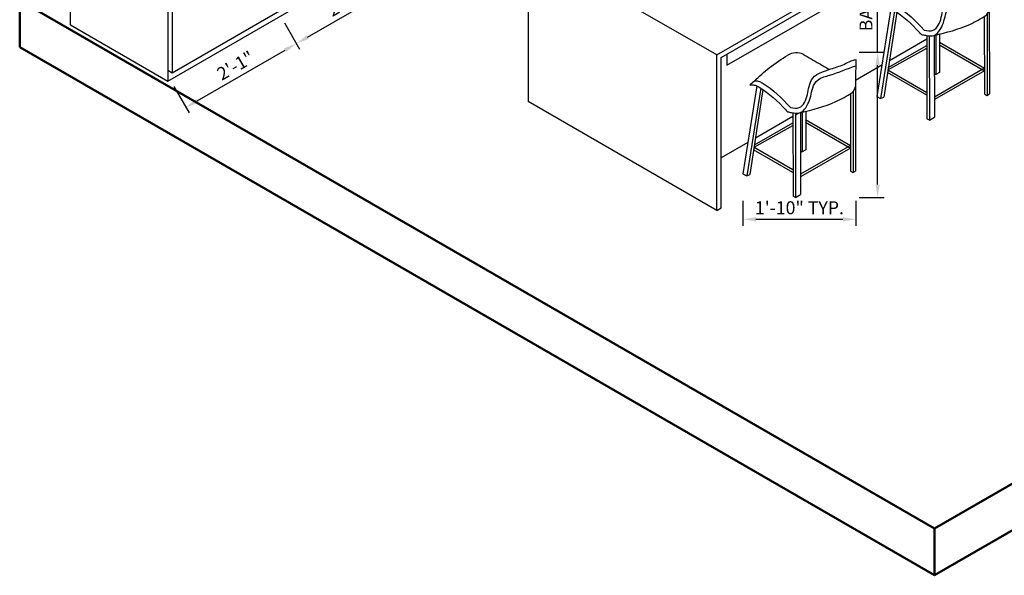
# Model space of a CAD drawing. Units: inches. Extents: x 5770 to 11891, y 3254 to 6808.
# Tile 1 of 15: x 5786 to 5976, y 3254 to 3361. Entities that reach past the tile are written whole.
import ezdxf

# ---------------------------------------------------------------- set-up
doc = ezdxf.new("R2010")
doc.units = ezdxf.units.IN
for name, color, linetype, lineweight in [('A-ANNO-DIMS', 2, 'Continuous', 18), ('A-FURN', 8, 'Continuous', 25), ('A-WALL', 7, 'Continuous', 50)]:
    doc.layers.add(name, color=color, linetype=linetype, lineweight=lineweight)
doc.styles.get("Standard").update_dxf_attribs({"font": 'arial.ttf'})
doc.dimstyles.new('ISO-25', dxfattribs={"dimtxt": 2.5, "dimasz": 2.5, "dimexe": 1.25, "dimexo": 0.625, "dimtad": 1, "dimdec": 0, "dimlunit": 3, "dimtxsty": 'Standard', "dimcen": 2.5, "dimadec": 0, "dimazin": 0, "dimtfac": 1, "dimtdec": 0, "dimtmove": 0, "dimatfit": 3, "dimfxl": 1, "dimarcsym": 0})

# ---------------------------------------------------------------- blocks, each defined once
blk = doc.blocks.new('*D1')
at = {"layer": 'A-ANNO-DIMS', "color": 0, "lineweight": -2, "transparency": 16777216}
for p, q in [((5837.13, 3360.58), (5840.08, 3355.46)), ((5820.33, 3345.5), (5837.29, 3355.29)), ((5815.83, 3348.29), (5818.79, 3343.17))]:
    blk.add_line(p, q, dxfattribs=at)
at = {"layer": 'A-ANNO-DIMS', "color": 0, "transparency": 16777216}
for points in [[(5837.08, 3355.65), (5837.5, 3354.93), (5839.46, 3356.54)], [(5820.12, 3345.86), (5820.54, 3345.14), (5818.16, 3344.25)]]:
    blk.add_solid(points, dxfattribs=at)
at = {"layer": 'Defpoints', "color": 0, "transparency": 16777216}
for p in [(5836.81, 3361.12), (5839.46, 3356.54), (5815.52, 3348.83)]:
    blk.add_point(p, dxfattribs=at)
at = {"layer": 'A-ANNO-DIMS', "color": 0, "transparency": 16777216, "insert": (5827.87, 3352.03), "char_height": 2.5, "attachment_point": 5, "rotation": 30}
blk.add_mtext('2\'-1"', dxfattribs=at)
blk = doc.blocks.new('*D2')
at = {"layer": 'A-ANNO-DIMS', "color": 0, "lineweight": -2, "transparency": 16777216}
for p, q in [((5858.42, 3372.87), (5861.37, 3367.75)), ((5841.62, 3357.79), (5858.58, 3367.59)), ((5837.13, 3360.58), (5840.08, 3355.46))]:
    blk.add_line(p, q, dxfattribs=at)
at = {"layer": 'A-ANNO-DIMS', "color": 0, "transparency": 16777216}
for points in [[(5858.37, 3367.95), (5858.79, 3367.23), (5860.75, 3368.84)], [(5841.41, 3358.15), (5841.83, 3357.43), (5839.46, 3356.54)]]:
    blk.add_solid(points, dxfattribs=at)
at = {"layer": 'Defpoints', "color": 0, "transparency": 16777216}
for p in [(5858.1, 3373.41), (5860.75, 3368.84), (5836.81, 3361.12)]:
    blk.add_point(p, dxfattribs=at)
at = {"layer": 'A-ANNO-DIMS', "color": 0, "transparency": 16777216, "insert": (5849.16, 3364.32), "char_height": 2.5, "attachment_point": 5, "rotation": 30}
blk.add_mtext('2\'-1"', dxfattribs=at)
blk = doc.blocks.new('CHAIR')
for p, q in [((5928.22, 3348.4), (5925.54, 3331.45)), ((5947.21, 3348.3), (5947.24, 3331.95)), ((5928.97, 3347.97), (5926.27, 3331.03)), ((5929.39, 3347.7), (5926.87, 3331.3)), ((5946.25, 3346.87), (5946.28, 3331.94)), ((5946.78, 3347.31), (5946.81, 3331.7)), ((5935.16, 3343.21), (5935.19, 3327.16)), ((5935.65, 3343.13), (5935.69, 3326.87)), ((5936.61, 3343.23), (5936.64, 3327.43)), ((5936.93, 3343.31), (5936.93, 3335.67)), ((5937.63, 3343.48), (5937.63, 3336.08)), ((5927.68, 3336.56), (5935.16, 3340.78)), ((5927.75, 3337.02), (5935.16, 3341.28)), ((5937.62, 3341.89), (5946.27, 3336.9)), ((5937.62, 3341.39), (5946.27, 3336.4)), ((5946.27, 3336.9), (5936.64, 3331.34)), ((5935.18, 3331.68), (5927.6, 3336.05)), ((5935.18, 3332.18), (5927.67, 3336.51)), ((5936.63, 3335.85), (5936.93, 3335.67)), ((5946.27, 3336.4), (5936.64, 3330.84)), ((5937.63, 3336.08), (5936.93, 3335.67)), ((5925.54, 3331.45), (5926.27, 3331.03)), ((5926.27, 3331.03), (5926.87, 3331.3)), ((5946.28, 3331.94), (5946.75, 3331.67)), ((5946.75, 3331.67), (5947.24, 3331.95)), ((5935.69, 3326.87), (5936.64, 3327.43)), ((5935.69, 3326.87), (5935.19, 3327.16))]:
    blk.add_line(p, q)
blk.add_arc((5935.85, 3351.36), 3.39, 67.7359, 118.7768)
for points, knots in [([(5926.85, 3348.57), (5927.14, 3348.84), (5927.44, 3349.11), (5927.74, 3349.38), (5928.67, 3350.23), (5930.69, 3352.07), (5932.98, 3353.56), (5934.22, 3354.33)], [-1.200535, -1.200535, -1.200535, -1.200535, 0, 0, 0, 3.797995, 8.17369, 8.17369, 8.17369, 8.17369]), ([(5937.14, 3354.49), (5938.17, 3353.9), (5939.86, 3352.92), (5941.54, 3351.95), (5942.19, 3351.57)], [1.567957, 1.567957, 1.567957, 1.567957, 5.157778, 7.408601, 7.408601, 7.408601, 7.408601]), ([(5934.12, 3343.4), (5934.38, 3343.35), (5934.65, 3343.3), (5934.92, 3343.25), (5935.52, 3343.14), (5936.61, 3342.93), (5938.16, 3344.68), (5938.85, 3347.35), (5939.3, 3349.5), (5941.12, 3350.13), (5941.47, 3350.25), (5941.87, 3350.35), (5942.28, 3350.46), (5944.02, 3351.01), (5945.63, 3351.73), (5947.28, 3352.25)], [-0.758098, -0.758098, -0.758098, -0.758098, 0, 0, 0, 1.699756, 3.089131, 6.324639, 10.056959, 10.056959, 10.056959, 10.772274, 10.772274, 10.772274, 13.697346, 13.697346, 13.697346, 13.697346]), ([(5940.89, 3351.1), (5941.41, 3351.3), (5942.76, 3351.79), (5944.67, 3352.3), (5946.17, 3353.17), (5946.99, 3353.38), (5947.3, 3353.46)], [0, 0, 0, 0, 1.664278, 4.310629, 5.889247, 6.833724, 6.833724, 6.833724, 6.833724]), ([(5947.3, 3353.46), (5947.28, 3352.49), (5947.26, 3351.53), (5947.25, 3350.57), (5947.24, 3350.2), (5947.23, 3349.82), (5947.23, 3349.45), (5947.22, 3349.07), (5947.21, 3348.69), (5947.21, 3348.3)], [0, 0, 0, 0, 2.886502, 2.886502, 2.886502, 4.003886, 4.003886, 4.003886, 5.15459, 5.15459, 5.15459, 5.15459]), ([(5934.69, 3344.22), (5935.29, 3344.11), (5936.38, 3343.91), (5937.93, 3345.66), (5938.13, 3348.59), (5939.07, 3350.47), (5940.89, 3351.1)], [0, 0, 0, 0, 1.699756, 3.089131, 6.324639, 10.056959, 10.056959, 10.056959, 10.056959]), ([(5926.85, 3348.57), (5926.95, 3348.57), (5927.05, 3348.57), (5927.15, 3348.57), (5927.4, 3348.57), (5927.95, 3348.58), (5930.42, 3347.16), (5932.26, 3345.42), (5933.78, 3343.76), (5933.78, 3343.76), (5933.79, 3343.75), (5933.79, 3343.75), (5933.9, 3343.63), (5934.01, 3343.51), (5934.12, 3343.4)], [-0.293735, -0.293735, -0.293735, -0.293735, 0, 0, 0, 0.763361, 1.613257, 8.34273, 8.34273, 8.34273, 8.363036, 8.363036, 8.363036, 8.838355, 8.838355, 8.838355, 8.838355]), ([(5927.74, 3349.38), (5928, 3349.38), (5928.54, 3349.38), (5931.15, 3347.89), (5933.07, 3346.01), (5934.69, 3344.22)], [0, 0, 0, 0, 0.763361, 1.613257, 8.813397, 8.813397, 8.813397, 8.813397]), ([(5946.61, 3347.1), (5946.8, 3347.33), (5947.08, 3347.7), (5947.18, 3348.14), (5947.21, 3348.3)], [0, 0, 0, 0, 0.871891, 1.360739, 1.360739, 1.360739, 1.360739]), ([(5936.62, 3343.23), (5938.95, 3343.8), (5942.47, 3344.66), (5945.58, 3346.46), (5946.61, 3347.1)], [0, 0, 0, 0, 7.14919, 10.770772, 10.770772, 10.770772, 10.770772])]:
    blk.add_open_spline(points, degree=3, knots=knots)
blk = doc.blocks.new('*D26')
at = {"layer": 'A-ANNO-DIMS', "color": 0, "lineweight": -2, "transparency": 16777216}
for p, q in [((5951.5, 3354.88), (5951.5, 3394.72)), ((5947.92, 3354.88), (5952.75, 3354.88)), ((5951.5, 3329.37), (5951.5, 3352.38)), ((5947.92, 3326.87), (5952.75, 3326.87))]:
    blk.add_line(p, q, dxfattribs=at)
at = {"layer": 'A-ANNO-DIMS', "color": 0, "transparency": 16777216}
for points in [[(5951.08, 3352.38), (5951.91, 3352.38), (5951.5, 3354.88)], [(5951.08, 3329.37), (5951.91, 3329.37), (5951.5, 3326.87)]]:
    blk.add_solid(points, dxfattribs=at)
at = {"layer": 'Defpoints', "color": 0, "transparency": 16777216}
for p in [(5947.3, 3354.88), (5951.5, 3354.88), (5947.3, 3326.87)]:
    blk.add_point(p, dxfattribs=at)
at = {"layer": 'A-ANNO-DIMS', "color": 0, "transparency": 16777216, "insert": (5949.58, 3376.05), "char_height": 2.5, "attachment_point": 5, "rotation": 90}
blk.add_mtext('BAR STOOL 2\'-4" TYP.', dxfattribs=at)
blk = doc.blocks.new('*D27')
at = {"layer": 'A-ANNO-DIMS', "color": 0, "lineweight": -2, "transparency": 16777216}
for p, q in [((5925.54, 3326.25), (5925.54, 3321.42)), ((5947.3, 3326.25), (5947.3, 3321.42)), ((5928.04, 3322.67), (5944.8, 3322.67))]:
    blk.add_line(p, q, dxfattribs=at)
at = {"layer": 'A-ANNO-DIMS', "color": 0, "transparency": 16777216}
for points in [[(5928.04, 3323.09), (5928.04, 3322.26), (5925.54, 3322.67)], [(5944.8, 3323.09), (5944.8, 3322.26), (5947.3, 3322.67)]]:
    blk.add_solid(points, dxfattribs=at)
at = {"layer": 'Defpoints', "color": 0, "transparency": 16777216}
for p in [(5925.54, 3326.87), (5947.3, 3326.87), (5947.3, 3322.67)]:
    blk.add_point(p, dxfattribs=at)
at = {"layer": 'A-ANNO-DIMS', "color": 0, "transparency": 16777216, "insert": (5936.42, 3324.57), "char_height": 2.5, "attachment_point": 5}
blk.add_mtext('1\'-10" TYP.', dxfattribs=at)

msp = doc.modelspace()

# ---------------------------------------------------------------- linework, layer by layer
at = {"layer": 'A-FURN'}
for p, q in [((5920.5, 3354.37), (6003.63, 3402.37)), ((5921.36, 3353.87), (6002.77, 3400.87)), ((5922.46, 3352.37), (5996.03, 3394.84)), ((5795.91, 3360.15), (5795.91, 3392.22)), ((5879.96, 3388.14), (5815.52, 3350.85)), ((5814.66, 3381.4), (5814.66, 3349.33)), ((5815.52, 3380.9), (5815.52, 3350.85)), ((5920.5, 3354.37), (5884.12, 3375.37)), ((5884.12, 3375.37), (5884.12, 3345.37)), ((5814.66, 3349.33), (5857.18, 3373.88)), ((5795.91, 3360.15), (5814.66, 3349.33)), ((5960.97, 3357.39), (5953.76, 3353.23)), ((5920.5, 3324.37), (5920.5, 3354.37)), ((5922.46, 3354.5), (5922.46, 3352.37)), ((5921.36, 3324.87), (5921.36, 3353.87)), ((5952.31, 3352.39), (5947.23, 3349.45)), ((5815.52, 3350.85), (5814.66, 3351.35)), ((5920.5, 3324.37), (5884.12, 3345.37)), ((5936.3, 3343.14), (5935.65, 3342.77)), ((5935.16, 3342.49), (5927.95, 3338.32)), ((5926.5, 3337.48), (5921.36, 3334.52)), ((5920.5, 3324.37), (5921.36, 3324.87))]:
    msp.add_line(p, q, dxfattribs=at)
at = {"layer": 'A-WALL'}
for p, q in [((5962.44, 3263.03), (5786.11, 3364.83)), ((5786.11, 3364.83), (5786.11, 3355.83)), ((5962.44, 3254.03), (5786.11, 3355.83)), ((6132.52, 3352.22), (5962.44, 3254.03)), ((6090.78, 3337.13), (5962.44, 3263.03)), ((5962.44, 3263.03), (5962.44, 3254.03))]:
    msp.add_line(p, q, dxfattribs=at)

# ---------------------------------------------------------------- block references
at = {"layer": 'A-FURN'}
for p in [(25.81, 14.9), (0, 0)]:
    msp.add_blockref('CHAIR', p, dxfattribs=at)

# ---------------------------------------------------------------- dimensions: what is measured, and where the dimension line sits
at = {"layer": 'A-ANNO-DIMS'}
dim = msp.add_linear_dim(base=(5951.5, 3354.88), p1=(5947.3, 3326.87), p2=(5947.3, 3354.88), angle=90, text='BAR STOOL <> TYP.', dimstyle='ISO-25', override={"dimdec": 1, "dimlfac": 1, "dimrnd": 0, "dimzin": 1, "dimdsep": 46, "dimlunit": 4, "dimfrac": 2}, dxfattribs=at)
dim.commit()
dim.dimension.update_dxf_attribs({"geometry": '*D26', "text_midpoint": (5949.58, 3376.05)})
for p1, p2, picture, middle in [((5836.81, 3361.12), (5858.1, 3373.41), '*D2', (5849.16, 3364.32)), ((5815.52, 3348.83), (5836.81, 3361.12), '*D1', (5827.87, 3352.03))]:
    dim = msp.add_aligned_dim(p1=p1, p2=p2, distance=-5.29, dimstyle='ISO-25', override={"dimclrd": 0, "dimclre": 0, "dimclrt": 0}, dxfattribs=at)
    dim.commit()
    dim.dimension.update_dxf_attribs({"geometry": picture, "text_midpoint": middle})
dim = msp.add_linear_dim(base=(5947.3, 3322.67), p1=(5925.54, 3326.87), p2=(5947.3, 3326.87), text='<> TYP.', dimstyle='ISO-25', override={"dimdec": 1, "dimlfac": 1, "dimrnd": 0, "dimzin": 1, "dimdsep": 46, "dimlunit": 4, "dimfrac": 2}, dxfattribs=at)
dim.commit()
dim.dimension.update_dxf_attribs({"geometry": '*D27', "text_midpoint": (5936.42, 3324.57)})

doc.saveas('drawing.dxf')
